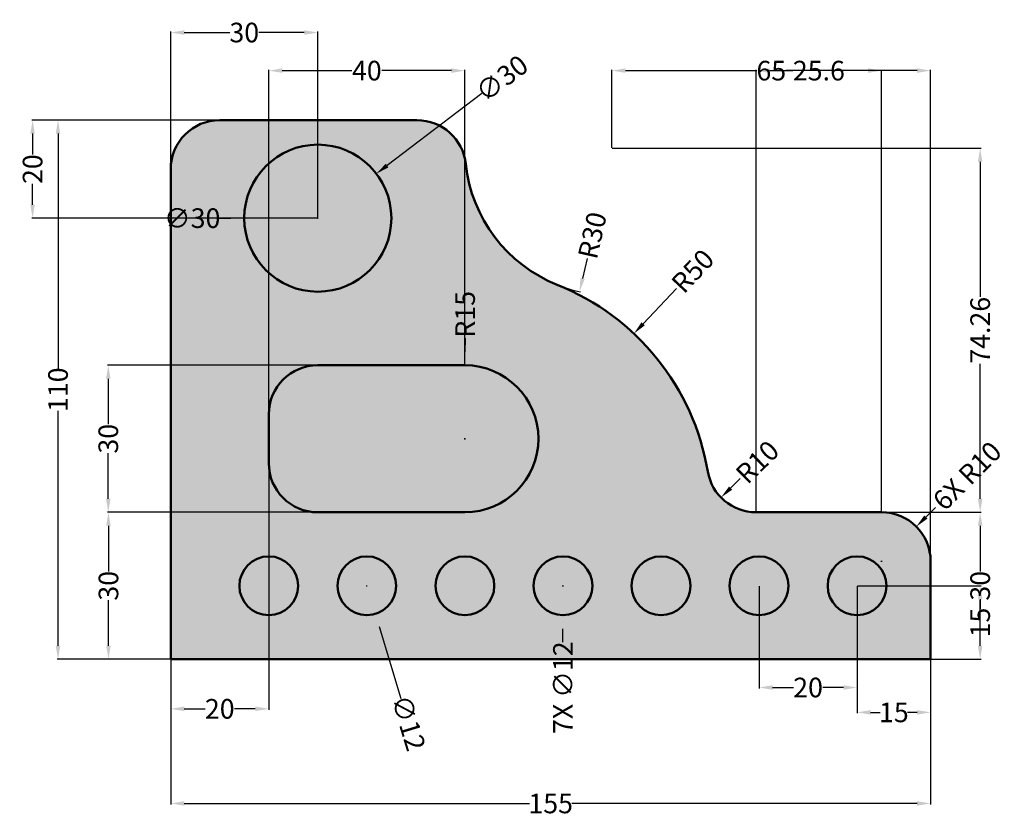
# Model space of a CAD drawing. Units: millimetres. Extents: x 347 to 548, y 156 to 318.
import ezdxf

# ---------------------------------------------------------------- set-up
doc = ezdxf.new("R2010")
doc.units = ezdxf.units.MM
doc.header["$MEASUREMENT"] = 0
doc.layers.add('M-DIMS', color=6, linetype='Continuous', lineweight=25)
doc.layers.add('M-OUTL', color=250, linetype='Continuous', lineweight=50)
doc.layers.add('M-HATC', color=252, linetype='Continuous', lineweight=18, true_color=0x939598)
doc.layers.add('M-HATC-OPENINGS', color=41, linetype='Continuous', lineweight=18, true_color=0xf4ee51)
doc.styles.get("Standard").update_dxf_attribs({"font": 'arial.ttf'})
doc.dimstyles.get("Standard").update_dxf_attribs({"dimtxt": 4, "dimasz": 2.75, "dimexe": 0.18, "dimexo": 0.0625, "dimgap": 0.09, "dimtad": 0, "dimdec": 0, "dimzin": 0, "dimdsep": 46, "dimtxsty": 'Standard', "dimcen": 0.09, "dimadec": 0, "dimazin": 0, "dimtfac": 1, "dimtdec": 0, "dimtofl": 0, "dimtmove": 0, "dimatfit": 3, "dimfxl": 1, "dimtolj": 1, "dimtzin": 0, "dimarcsym": 0})

# ---------------------------------------------------------------- blocks, each defined once
blk = doc.blocks.new('*D1')
at = {"layer": 'Defpoints', "color": 0, "transparency": 16777216}
for p in [(422.92, 217.89), (365.22, 187.89), (422.92, 187.89)]:
    blk.add_point(p, dxfattribs=at)
at = {"layer": 'M-DIMS', "color": 0, "lineweight": -2, "transparency": 16777216}
for p, q in [((422.85, 217.89), (365.04, 217.89)), ((365.22, 215.14), (365.22, 205.83)), ((365.22, 190.64), (365.22, 199.94)), ((422.85, 187.89), (365.04, 187.89))]:
    blk.add_line(p, q, dxfattribs=at)
at = {"layer": 'M-DIMS', "color": 0, "transparency": 16777216}
for points in [[(364.76, 215.14), (365.67, 215.14), (365.22, 217.89)], [(364.76, 190.64), (365.67, 190.64), (365.22, 187.89)]]:
    blk.add_solid(points, dxfattribs=at)
at = {"layer": 'M-DIMS', "color": 0, "transparency": 16777216, "insert": (365.22, 202.89), "char_height": 4, "attachment_point": 5, "rotation": 90}
blk.add_mtext('\\A1;30', dxfattribs=at)
blk = doc.blocks.new('*D2')
at = {"layer": 'Defpoints', "color": 0, "transparency": 16777216}
for p in [(365.18, 247.89), (422.92, 247.89), (422.92, 217.89)]:
    blk.add_point(p, dxfattribs=at)
at = {"layer": 'M-DIMS', "color": 0, "lineweight": -2, "transparency": 16777216}
for p, q in [((422.85, 247.89), (365, 247.89)), ((365.18, 245.14), (365.18, 235.83)), ((365.18, 220.64), (365.18, 229.94)), ((422.85, 217.89), (365, 217.89))]:
    blk.add_line(p, q, dxfattribs=at)
at = {"layer": 'M-DIMS', "color": 0, "transparency": 16777216}
for points in [[(364.72, 245.14), (365.64, 245.14), (365.18, 247.89)], [(364.72, 220.64), (365.64, 220.64), (365.18, 217.89)]]:
    blk.add_solid(points, dxfattribs=at)
at = {"layer": 'M-DIMS', "color": 0, "transparency": 16777216, "insert": (365.18, 232.89), "char_height": 4, "attachment_point": 5, "rotation": 90}
blk.add_mtext('\\A1;30', dxfattribs=at)
blk = doc.blocks.new('*D3')
at = {"layer": 'Defpoints', "color": 0, "transparency": 16777216}
for p in [(349.74, 297.89), (408.03, 297.89), (407.92, 277.89)]:
    blk.add_point(p, dxfattribs=at)
at = {"layer": 'M-DIMS', "color": 0, "lineweight": -2, "transparency": 16777216}
for p, q in [((407.97, 297.89), (349.56, 297.89)), ((349.74, 295.14), (349.74, 290.87)), ((349.74, 280.64), (349.74, 284.9)), ((407.85, 277.89), (349.56, 277.89))]:
    blk.add_line(p, q, dxfattribs=at)
at = {"layer": 'M-DIMS', "color": 0, "transparency": 16777216}
for points in [[(349.28, 295.14), (350.19, 295.14), (349.74, 297.89)], [(349.28, 280.64), (350.19, 280.64), (349.74, 277.89)]]:
    blk.add_solid(points, dxfattribs=at)
at = {"layer": 'M-DIMS', "color": 0, "transparency": 16777216, "insert": (349.74, 287.89), "char_height": 4, "attachment_point": 5, "rotation": 90}
blk.add_mtext('\\A1;20', dxfattribs=at)
blk = doc.blocks.new('*D4')
at = {"layer": 'Defpoints', "color": 0, "transparency": 16777216}
for p in [(407.92, 315.76), (377.92, 277.89), (407.92, 277.89)]:
    blk.add_point(p, dxfattribs=at)
at = {"layer": 'M-DIMS', "color": 0, "lineweight": -2, "transparency": 16777216}
for p, q in [((377.92, 277.95), (377.92, 315.94)), ((380.67, 315.76), (389.97, 315.76)), ((405.17, 315.76), (395.86, 315.76)), ((407.92, 277.95), (407.92, 315.94))]:
    blk.add_line(p, q, dxfattribs=at)
at = {"layer": 'M-DIMS', "color": 0, "transparency": 16777216}
for points in [[(380.67, 316.22), (380.67, 315.3), (377.92, 315.76)], [(405.17, 316.22), (405.17, 315.3), (407.92, 315.76)]]:
    blk.add_solid(points, dxfattribs=at)
at = {"layer": 'M-DIMS', "color": 0, "transparency": 16777216, "insert": (392.92, 315.76), "char_height": 4, "attachment_point": 5}
blk.add_mtext('\\A1;30', dxfattribs=at)
blk = doc.blocks.new('*D5')
at = {"layer": 'Defpoints', "color": 0, "transparency": 16777216}
for p in [(387.92, 297.89), (354.93, 187.89), (387.92, 187.89)]:
    blk.add_point(p, dxfattribs=at)
at = {"layer": 'M-DIMS', "color": 0, "lineweight": -2, "transparency": 16777216}
for p, q in [((387.85, 297.89), (354.75, 297.89)), ((354.93, 295.14), (354.93, 247.2)), ((354.93, 190.64), (354.93, 238.57)), ((387.85, 187.89), (354.75, 187.89))]:
    blk.add_line(p, q, dxfattribs=at)
at = {"layer": 'M-DIMS', "color": 0, "transparency": 16777216}
for points in [[(354.47, 295.14), (355.39, 295.14), (354.93, 297.89)], [(354.47, 190.64), (355.39, 190.64), (354.93, 187.89)]]:
    blk.add_solid(points, dxfattribs=at)
at = {"layer": 'M-DIMS', "color": 0, "transparency": 16777216, "insert": (354.93, 242.89), "char_height": 4, "attachment_point": 5, "rotation": 90}
blk.add_mtext('\\A1;110', dxfattribs=at)
blk = doc.blocks.new('*D6')
at = {"layer": 'Defpoints', "color": 0, "transparency": 16777216}
for p in [(419.86, 286.96), (395.97, 268.81)]:
    blk.add_point(p, dxfattribs=at)
at = {"layer": 'M-DIMS', "color": 0, "lineweight": -2, "transparency": 16777216}
for p, q in [((441.38, 303.31), (422.05, 288.63)), ((407.83, 277.89), (408.01, 277.89)), ((407.92, 277.8), (407.92, 277.98))]:
    blk.add_line(p, q, dxfattribs=at)
at = {"layer": 'M-DIMS', "color": 0, "transparency": 16777216}
blk.add_solid([(421.77, 288.99), (422.33, 288.26), (419.86, 286.96)], dxfattribs=at)
at = {"layer": 'M-DIMS', "color": 0, "transparency": 16777216, "insert": (445.46, 306.41), "char_height": 4, "attachment_point": 5, "rotation": 37.2288}
blk.add_mtext('\\A1;∅30', dxfattribs=at)
blk = doc.blocks.new('*D7')
at = {"layer": 'Defpoints', "color": 0, "transparency": 16777216}
for p in [(467.92, 292.15), (461.31, 262.88)]:
    blk.add_point(p, dxfattribs=at)
at = {"layer": 'M-DIMS', "color": 0, "lineweight": -2, "transparency": 16777216}
blk.add_line((462.84, 269.63), (461.92, 265.56), dxfattribs=at)
blk.add_arc((467.92, 292.15), 30, 248.2811, 257.6241, dxfattribs=at)
at = {"layer": 'M-DIMS', "color": 0, "transparency": 16777216}
blk.add_solid([(461.47, 265.67), (462.36, 265.46), (461.31, 262.88)], dxfattribs=at)
at = {"layer": 'M-DIMS', "color": 0, "transparency": 16777216, "insert": (463.91, 274.38), "char_height": 4, "attachment_point": 5, "rotation": 77.2804}
blk.add_mtext('\\A1;R30', dxfattribs=at)
blk = doc.blocks.new('*D8')
at = {"layer": 'Defpoints', "color": 0, "transparency": 16777216}
for p in [(472.39, 254.33), (438.16, 217.89)]:
    blk.add_point(p, dxfattribs=at)
at = {"layer": 'M-DIMS', "color": 0, "lineweight": -2, "transparency": 16777216}
for p, q in [((481.06, 263.56), (474.27, 256.33)), ((438.07, 217.89), (438.25, 217.89)), ((438.16, 217.8), (438.16, 217.98))]:
    blk.add_line(p, q, dxfattribs=at)
at = {"layer": 'M-DIMS', "color": 0, "transparency": 16777216}
blk.add_solid([(473.94, 256.65), (474.61, 256.02), (472.39, 254.33)], dxfattribs=at)
at = {"layer": 'M-DIMS', "color": 0, "transparency": 16777216, "insert": (484.39, 267.11), "char_height": 4, "attachment_point": 5, "rotation": 46.7913}
blk.add_mtext('\\A1;R50', dxfattribs=at)
blk = doc.blocks.new('*D9')
at = {"layer": 'Defpoints', "color": 0, "transparency": 16777216}
for p in [(497.32, 227.89), (490.16, 220.91)]:
    blk.add_point(p, dxfattribs=at)
at = {"layer": 'M-DIMS', "color": 0, "lineweight": -2, "transparency": 16777216}
blk.add_line((494.1, 224.75), (492.13, 222.83), dxfattribs=at)
at = {"layer": 'M-DIMS', "color": 0, "transparency": 16777216}
blk.add_solid([(491.81, 223.15), (492.45, 222.5), (490.16, 220.91)], dxfattribs=at)
at = {"layer": 'M-DIMS', "color": 0, "transparency": 16777216, "insert": (497.58, 228.14), "char_height": 4, "attachment_point": 5, "rotation": 44.268}
blk.add_mtext('\\A1;R10', dxfattribs=at)
blk = doc.blocks.new('*D10')
at = {"layer": 'Defpoints', "color": 0, "transparency": 16777216}
for p in [(497.92, 202.89), (517.92, 202.89), (517.92, 182.14)]:
    blk.add_point(p, dxfattribs=at)
at = {"layer": 'M-DIMS', "color": 0, "lineweight": -2, "transparency": 16777216}
for p, q in [((497.92, 202.82), (497.92, 181.96)), ((517.92, 202.82), (517.92, 181.96)), ((500.67, 182.14), (504.94, 182.14)), ((515.17, 182.14), (510.9, 182.14))]:
    blk.add_line(p, q, dxfattribs=at)
at = {"layer": 'M-DIMS', "color": 0, "transparency": 16777216}
for points in [[(500.67, 182.59), (500.67, 181.68), (497.92, 182.14)], [(515.17, 182.59), (515.17, 181.68), (517.92, 182.14)]]:
    blk.add_solid(points, dxfattribs=at)
at = {"layer": 'M-DIMS', "color": 0, "transparency": 16777216, "insert": (507.92, 182.14), "char_height": 4, "attachment_point": 5}
blk.add_mtext('\\A1;20', dxfattribs=at)
blk = doc.blocks.new('*D11')
at = {"layer": 'Defpoints', "color": 0, "transparency": 16777216}
for p in [(517.92, 202.89), (532.92, 202.89), (532.92, 177.06)]:
    blk.add_point(p, dxfattribs=at)
at = {"layer": 'M-DIMS', "color": 0, "lineweight": -2, "transparency": 16777216}
for p, q in [((517.92, 202.82), (517.92, 176.88)), ((532.92, 202.82), (532.92, 176.88)), ((520.67, 177.06), (522.64, 177.06)), ((530.17, 177.06), (528.2, 177.06))]:
    blk.add_line(p, q, dxfattribs=at)
at = {"layer": 'M-DIMS', "color": 0, "transparency": 16777216}
for points in [[(520.67, 177.52), (520.67, 176.6), (517.92, 177.06)], [(530.17, 177.52), (530.17, 176.6), (532.92, 177.06)]]:
    blk.add_solid(points, dxfattribs=at)
at = {"layer": 'M-DIMS', "color": 0, "transparency": 16777216, "insert": (525.42, 177.06), "char_height": 4, "attachment_point": 5}
blk.add_mtext('\\A1;15', dxfattribs=at)
blk = doc.blocks.new('*D12')
at = {"layer": 'Defpoints', "color": 0, "transparency": 16777216}
for p in [(377.92, 187.89), (532.92, 187.89), (532.92, 158.48)]:
    blk.add_point(p, dxfattribs=at)
at = {"layer": 'M-DIMS', "color": 0, "lineweight": -2, "transparency": 16777216}
for p, q in [((377.92, 187.82), (377.92, 158.3)), ((532.92, 187.82), (532.92, 158.3)), ((380.67, 158.48), (451.08, 158.48)), ((530.17, 158.48), (459.75, 158.48))]:
    blk.add_line(p, q, dxfattribs=at)
at = {"layer": 'M-DIMS', "color": 0, "transparency": 16777216}
for points in [[(380.67, 158.94), (380.67, 158.03), (377.92, 158.48)], [(530.17, 158.94), (530.17, 158.03), (532.92, 158.48)]]:
    blk.add_solid(points, dxfattribs=at)
at = {"layer": 'M-DIMS', "color": 0, "transparency": 16777216, "insert": (455.42, 158.48), "char_height": 4, "attachment_point": 5}
blk.add_mtext('\\A1;155', dxfattribs=at)
blk = doc.blocks.new('*D13')
at = {"layer": 'Defpoints', "color": 0, "transparency": 16777216}
for p in [(416.17, 208.63), (419.67, 197.15)]:
    blk.add_point(p, dxfattribs=at)
at = {"layer": 'M-DIMS', "color": 0, "lineweight": -2, "transparency": 16777216}
for p, q in [((417.83, 202.89), (418.01, 202.89)), ((417.92, 202.8), (417.92, 202.98)), ((424.95, 179.8), (420.47, 194.52))]:
    blk.add_line(p, q, dxfattribs=at)
at = {"layer": 'M-DIMS', "color": 0, "transparency": 16777216}
blk.add_solid([(420.91, 194.65), (420.03, 194.38), (419.67, 197.15)], dxfattribs=at)
at = {"layer": 'M-DIMS', "color": 0, "transparency": 16777216, "insert": (426.44, 174.91), "char_height": 4, "attachment_point": 5, "rotation": 286.9446}
blk.add_mtext('\\A1;∅12', dxfattribs=at)
blk = doc.blocks.new('FLANGE-HOLE-D12')
blk.add_circle((6, 6), 6)
blk = doc.blocks.new('*D15')
at = {"layer": 'Defpoints', "color": 0, "transparency": 16777216}
for p in [(517.92, 202.89), (532.92, 187.89), (543.02, 187.89)]:
    blk.add_point(p, dxfattribs=at)
at = {"layer": 'M-DIMS', "color": 0, "lineweight": -2, "transparency": 16777216}
for p, q in [((517.98, 202.89), (543.2, 202.89)), ((543.02, 200.14), (543.02, 198.17)), ((543.02, 190.64), (543.02, 192.61)), ((532.98, 187.89), (543.2, 187.89))]:
    blk.add_line(p, q, dxfattribs=at)
at = {"layer": 'M-DIMS', "color": 0, "transparency": 16777216}
for points in [[(542.56, 200.14), (543.48, 200.14), (543.02, 202.89)], [(542.56, 190.64), (543.48, 190.64), (543.02, 187.89)]]:
    blk.add_solid(points, dxfattribs=at)
at = {"layer": 'M-DIMS', "color": 0, "transparency": 16777216, "insert": (543.02, 195.39), "char_height": 4, "attachment_point": 5, "rotation": 90}
blk.add_mtext('\\A1;15', dxfattribs=at)
blk = doc.blocks.new('*D16')
at = {"layer": 'Defpoints', "color": 0, "transparency": 16777216}
for p in [(397.92, 227.89), (377.92, 187.89), (397.92, 177.79)]:
    blk.add_point(p, dxfattribs=at)
at = {"layer": 'M-DIMS', "color": 0, "lineweight": -2, "transparency": 16777216}
for p, q in [((397.92, 227.82), (397.92, 177.61)), ((377.92, 187.82), (377.92, 177.61)), ((380.67, 177.79), (384.94, 177.79)), ((395.17, 177.79), (390.9, 177.79))]:
    blk.add_line(p, q, dxfattribs=at)
at = {"layer": 'M-DIMS', "color": 0, "transparency": 16777216}
for points in [[(380.67, 178.25), (380.67, 177.33), (377.92, 177.79)], [(395.17, 178.25), (395.17, 177.33), (397.92, 177.79)]]:
    blk.add_solid(points, dxfattribs=at)
at = {"layer": 'M-DIMS', "color": 0, "transparency": 16777216, "insert": (387.92, 177.79), "char_height": 4, "attachment_point": 5}
blk.add_mtext('\\A1;20', dxfattribs=at)
blk = doc.blocks.new('*D17')
at = {"layer": 'Defpoints', "color": 0, "transparency": 16777216}
for p in [(437.92, 307.99), (437.92, 247.89), (397.92, 237.89)]:
    blk.add_point(p, dxfattribs=at)
at = {"layer": 'M-DIMS', "color": 0, "lineweight": -2, "transparency": 16777216}
for p, q in [((397.92, 237.95), (397.92, 308.17)), ((400.67, 307.99), (414.89, 307.99)), ((435.17, 307.99), (420.95, 307.99)), ((437.92, 247.95), (437.92, 308.17))]:
    blk.add_line(p, q, dxfattribs=at)
at = {"layer": 'M-DIMS', "color": 0, "transparency": 16777216}
for points in [[(400.67, 308.45), (400.67, 307.53), (397.92, 307.99)], [(435.17, 308.45), (435.17, 307.53), (437.92, 307.99)]]:
    blk.add_solid(points, dxfattribs=at)
at = {"layer": 'M-DIMS', "color": 0, "transparency": 16777216, "insert": (417.92, 307.99), "char_height": 4, "attachment_point": 5}
blk.add_mtext('\\A1;40', dxfattribs=at)
blk = doc.blocks.new('*D18')
at = {"layer": 'Defpoints', "color": 0, "transparency": 16777216}
for p in [(522.92, 217.89), (532.92, 187.89), (543.02, 187.89)]:
    blk.add_point(p, dxfattribs=at)
at = {"layer": 'M-DIMS', "color": 0, "lineweight": -2, "transparency": 16777216}
for p, q in [((522.98, 217.89), (543.2, 217.89)), ((543.02, 215.14), (543.02, 205.83)), ((543.02, 190.64), (543.02, 199.94)), ((532.98, 187.89), (543.2, 187.89))]:
    blk.add_line(p, q, dxfattribs=at)
at = {"layer": 'M-DIMS', "color": 0, "transparency": 16777216}
for points in [[(542.56, 215.14), (543.48, 215.14), (543.02, 217.89)], [(542.56, 190.64), (543.48, 190.64), (543.02, 187.89)]]:
    blk.add_solid(points, dxfattribs=at)
at = {"layer": 'M-DIMS', "color": 0, "transparency": 16777216, "insert": (543.02, 202.89), "char_height": 4, "attachment_point": 5, "rotation": 90}
blk.add_mtext('\\A1;30', dxfattribs=at)
blk = doc.blocks.new('*D19')
at = {"layer": 'Defpoints', "color": 0, "transparency": 16777216}
for p in [(522.92, 307.99), (497.32, 217.89), (522.92, 217.89)]:
    blk.add_point(p, dxfattribs=at)
at = {"layer": 'M-DIMS', "color": 0, "lineweight": -2, "transparency": 16777216}
for p, q in [((497.32, 217.95), (497.32, 308.17)), ((500.07, 307.99), (504.8, 307.99)), ((520.17, 307.99), (515.44, 307.99)), ((522.92, 217.95), (522.92, 308.17))]:
    blk.add_line(p, q, dxfattribs=at)
at = {"layer": 'M-DIMS', "color": 0, "transparency": 16777216}
for points in [[(500.07, 308.45), (500.07, 307.53), (497.32, 307.99)], [(520.17, 308.45), (520.17, 307.53), (522.92, 307.99)]]:
    blk.add_solid(points, dxfattribs=at)
at = {"layer": 'M-DIMS', "color": 0, "transparency": 16777216, "insert": (510.12, 307.99), "char_height": 4, "attachment_point": 5}
blk.add_mtext('\\A1;25.6', dxfattribs=at)
blk = doc.blocks.new('*D20')
at = {"layer": 'Defpoints', "color": 0, "transparency": 16777216}
for p in [(532.92, 307.99), (467.92, 292.15), (532.92, 207.89)]:
    blk.add_point(p, dxfattribs=at)
at = {"layer": 'M-DIMS', "color": 0, "lineweight": -2, "transparency": 16777216}
for p, q in [((467.92, 292.21), (467.92, 308.17)), ((470.67, 307.99), (497.44, 307.99)), ((530.17, 307.99), (503.4, 307.99)), ((532.92, 207.95), (532.92, 308.17))]:
    blk.add_line(p, q, dxfattribs=at)
at = {"layer": 'M-DIMS', "color": 0, "transparency": 16777216}
for points in [[(470.67, 308.45), (470.67, 307.53), (467.92, 307.99)], [(530.17, 308.45), (530.17, 307.53), (532.92, 307.99)]]:
    blk.add_solid(points, dxfattribs=at)
at = {"layer": 'M-DIMS', "color": 0, "transparency": 16777216, "insert": (500.42, 307.99), "char_height": 4, "attachment_point": 5}
blk.add_mtext('\\A1;65', dxfattribs=at)
blk = doc.blocks.new('*D21')
at = {"layer": 'Defpoints', "color": 0, "transparency": 16777216}
for p in [(467.92, 292.15), (522.92, 217.89), (543.02, 217.89)]:
    blk.add_point(p, dxfattribs=at)
at = {"layer": 'M-DIMS', "color": 0, "lineweight": -2, "transparency": 16777216}
for p, q in [((467.98, 292.15), (543.2, 292.15)), ((543.02, 289.4), (543.02, 261.84)), ((543.02, 220.64), (543.02, 248.2)), ((522.98, 217.89), (543.2, 217.89))]:
    blk.add_line(p, q, dxfattribs=at)
at = {"layer": 'M-DIMS', "color": 0, "transparency": 16777216}
for points in [[(542.56, 289.4), (543.48, 289.4), (543.02, 292.15)], [(542.56, 220.64), (543.48, 220.64), (543.02, 217.89)]]:
    blk.add_solid(points, dxfattribs=at)
at = {"layer": 'M-DIMS', "color": 0, "transparency": 16777216, "insert": (543.02, 255.02), "char_height": 4, "attachment_point": 5, "rotation": 90}
blk.add_mtext('\\A1;74.26', dxfattribs=at)
blk = doc.blocks.new('*D22')
at = {"layer": 'Defpoints', "color": 0, "transparency": 16777216}
for p in [(392.92, 277.89), (422.92, 277.89)]:
    blk.add_point(p, dxfattribs=at)
at = {"layer": 'M-DIMS', "color": 0, "lineweight": -2, "transparency": 16777216}
for p, q in [((387.42, 277.89), (390.17, 277.89)), ((407.83, 277.89), (408.01, 277.89)), ((407.92, 277.8), (407.92, 277.98))]:
    blk.add_line(p, q, dxfattribs=at)
at = {"layer": 'M-DIMS', "color": 0, "transparency": 16777216}
blk.add_solid([(390.17, 278.35), (390.17, 277.43), (392.92, 277.89)], dxfattribs=at)
at = {"layer": 'M-DIMS', "color": 0, "transparency": 16777216, "insert": (382.29, 277.89), "char_height": 4, "attachment_point": 5, "rotation": 0.0002}
blk.add_mtext('\\A1;∅30', dxfattribs=at)
blk = doc.blocks.new('*D23')
at = {"layer": 'Defpoints', "color": 0, "transparency": 16777216}
for p in [(437.94, 247.89), (437.92, 232.89)]:
    blk.add_point(p, dxfattribs=at)
at = {"layer": 'M-DIMS', "color": 0, "lineweight": -2, "transparency": 16777216}
for p, q in [((437.95, 253.39), (437.94, 250.64)), ((437.92, 232.8), (437.92, 232.98)), ((437.83, 232.89), (438.01, 232.89))]:
    blk.add_line(p, q, dxfattribs=at)
at = {"layer": 'M-DIMS', "color": 0, "transparency": 16777216}
blk.add_solid([(437.49, 250.64), (438.4, 250.64), (437.94, 247.89)], dxfattribs=at)
at = {"layer": 'M-DIMS', "color": 0, "transparency": 16777216, "insert": (437.96, 258.27), "char_height": 4, "attachment_point": 5, "rotation": 89.9138}
blk.add_mtext('\\A1;R15', dxfattribs=at)
blk = doc.blocks.new('*D24')
at = {"layer": 'Defpoints', "color": 0, "transparency": 16777216}
for p in [(529.99, 214.96), (522.92, 207.89)]:
    blk.add_point(p, dxfattribs=at)
at = {"layer": 'M-DIMS', "color": 0, "lineweight": -2, "transparency": 16777216}
for p, q in [((533.88, 218.85), (531.93, 216.9)), ((522.83, 207.89), (523.01, 207.89)), ((522.92, 207.8), (522.92, 207.98))]:
    blk.add_line(p, q, dxfattribs=at)
at = {"layer": 'M-DIMS', "color": 0, "transparency": 16777216}
blk.add_solid([(531.61, 217.23), (532.26, 216.58), (529.99, 214.96)], dxfattribs=at)
at = {"layer": 'M-DIMS', "color": 0, "transparency": 16777216, "insert": (540.36, 225.33), "char_height": 4, "attachment_point": 5, "rotation": 45.0015}
blk.add_mtext('\\A1;6X R10', dxfattribs=at)
blk = doc.blocks.new('*D25')
at = {"layer": 'Defpoints', "color": 0, "transparency": 16777216}
for p in [(457.92, 208.89), (457.92, 196.89)]:
    blk.add_point(p, dxfattribs=at)
at = {"layer": 'M-DIMS', "color": 0, "lineweight": -2, "transparency": 16777216}
for p, q in [((457.83, 202.89), (458.01, 202.89)), ((457.92, 202.8), (457.92, 202.98)), ((457.92, 191.39), (457.92, 194.14))]:
    blk.add_line(p, q, dxfattribs=at)
at = {"layer": 'M-DIMS', "color": 0, "transparency": 16777216}
blk.add_solid([(457.46, 194.14), (458.38, 194.14), (457.92, 196.89)], dxfattribs=at)
at = {"layer": 'M-DIMS', "color": 0, "transparency": 16777216, "insert": (457.92, 182.1), "char_height": 4, "attachment_point": 5, "rotation": 89.996}
blk.add_mtext('\\A1;7X ∅12', dxfattribs=at)

msp = doc.modelspace()

# ---------------------------------------------------------------- hatches: boundary and pattern name
at = {"layer": 'M-HATC'}
h = msp.add_hatch(color=256, dxfattribs=at)
h.dxf.hatch_style = 1
h.paths.add_polyline_path([(456.758, 264.299, -0.2775575), (438.088, 288.952, 0.3833025), (428.145, 297.887), (387.917, 297.887, 0.4142136), (377.917, 287.887), (377.917, 187.887), (397.917, 187.887), (532.917, 187.887), (532.917, 207.887, 0.4142136), (522.917, 217.887), (497.319, 217.887, -0.3659774), (487.459, 226.22, 0.261262)])
h.paths.add_polyline_path([(407.917, 247.887), (437.917, 247.887, -1), (437.917, 217.887), (407.917, 217.887, -0.4142136), (397.917, 227.887), (397.917, 237.887, -0.4142136)], flags=16)
h.paths.add_polyline_path([(392.917, 277.887, -1), (422.917, 277.887, -1)], flags=16)
h.paths.add_polyline_path([(403.917, 202.887, -1), (391.917, 202.887, -1)], flags=16)
h.paths.add_polyline_path([(423.917, 202.887, -1), (411.917, 202.887, -1)], flags=16)
h.paths.add_polyline_path([(443.917, 202.887, -1), (431.917, 202.887, -1)], flags=16)
h.paths.add_polyline_path([(463.917, 202.887, -1), (451.917, 202.887, -1)], flags=16)
h.paths.add_polyline_path([(483.917, 202.887, -1), (471.917, 202.887, -1)], flags=16)
h.paths.add_polyline_path([(503.917, 202.887, -1), (491.917, 202.887, -1)], flags=16)
h.paths.add_polyline_path([(523.917, 202.887, -1), (511.917, 202.887, -1)], flags=16)
at = {"layer": 'M-HATC-OPENINGS'}
h = msp.add_hatch(color=256, dxfattribs=at)
h.dxf.hatch_style = 1
h.paths.add_polyline_path([(422.917, 277.887, 1), (392.917, 277.887, 1)])
h.paths.add_polyline_path([(437.917, 247.887), (407.917, 247.887, 0.4142136), (397.917, 237.887), (397.917, 232.887), (397.917, 227.887, 0.4142136), (407.917, 217.887), (437.917, 217.887, 1)])
h.paths.add_polyline_path([(391.917, 202.887, 1), (403.917, 202.887, 1)])
h.paths.add_polyline_path([(423.917, 202.887, 1), (411.917, 202.887, 1)])
h.paths.add_polyline_path([(443.917, 202.887, 1), (431.917, 202.887, 1)])
h.paths.add_polyline_path([(451.917, 202.887, 1), (463.917, 202.887, 1)])
h.paths.add_polyline_path([(483.917, 202.887, 1), (471.917, 202.887, 1)])
h.paths.add_polyline_path([(503.917, 202.887, 1), (491.917, 202.887, 1)])
h.paths.add_polyline_path([(523.917, 202.887, 1), (511.917, 202.887, 1)])

# ---------------------------------------------------------------- linework, layer by layer
at = {"layer": 'M-OUTL'}
for p, q in [((387.917, 297.887), (428.145, 297.887)), ((377.917, 187.887), (377.917, 287.887)), ((377.917, 287.887), (377.917, 187.887)), ((407.917, 247.887), (437.917, 247.887)), ((397.917, 232.887), (397.917, 237.887)), ((397.917, 227.887), (397.917, 237.887)), ((437.917, 217.887), (407.917, 217.887)), ((407.917, 217.887), (437.917, 217.887)), ((497.319, 217.887), (522.917, 217.887)), ((532.917, 187.887), (532.917, 207.887)), ((377.917, 187.887), (532.917, 187.887))]:
    msp.add_line(p, q, dxfattribs=at)
msp.add_circle((407.917, 277.887), 15, dxfattribs=at)
for centre, radius, start, end in [((387.917, 287.887), 10, 90, 180), ((428.145, 287.887), 10, 6.11219, 90), ((467.917, 292.146), 30, 186.11219, 248.16177), ((438.158, 217.887), 50, 9.59407, 68.16177), ((407.917, 237.887), 10, 90, 180), ((437.917, 232.887), 15, 270, 90), ((407.917, 227.887), 10, 180, 270), ((497.319, 227.887), 10, 189.59407, 270), ((522.917, 207.887), 10, 0, 90)]:
    msp.add_arc(centre, radius, start, end, dxfattribs=at)

# ---------------------------------------------------------------- block references
for p in [(391.917, 196.887), (411.917, 196.887), (431.917, 196.887), (451.917, 196.887), (471.917, 196.887), (491.917, 196.887), (511.917, 196.887)]:
    msp.add_blockref('FLANGE-HOLE-D12', p, dxfattribs=at)

# ---------------------------------------------------------------- dimensions: what is measured, and where the dimension line sits
at = {"layer": 'M-DIMS'}
for base, p1, p2, override, picture, middle in [((407.917, 315.757), (377.917, 277.887), (407.917, 277.887), {"dimclrd": 0, "dimclre": 0, "dimclrt": 0}, '*D4', (392.917, 315.757)), ((437.917, 307.987), (397.917, 237.887), (437.917, 247.887), {"dimdec": 0, "dimlfac": 1, "dimrnd": 0, "dimzin": 0, "dimdsep": 46, "dimlunit": 2}, '*D17', (417.917, 307.987)), ((532.917, 307.987), (467.917, 292.146), (532.917, 207.887), {"dimdec": 0, "dimlfac": 1, "dimrnd": 0, "dimzin": 0, "dimdsep": 46, "dimlunit": 2}, '*D20', (500.417, 307.987)), ((522.917, 307.987), (497.319, 217.887), (522.917, 217.887), {"dimdec": 1, "dimlfac": 1, "dimrnd": 0, "dimzin": 0, "dimdsep": 46, "dimlunit": 2}, '*D19', (510.118, 307.987)), ((397.917, 177.787), (377.917, 187.887), (397.917, 227.887), {"dimdec": 0, "dimlfac": 1, "dimrnd": 0, "dimzin": 0, "dimdsep": 46, "dimlunit": 2}, '*D16', (387.917, 177.787)), ((517.917, 182.136), (497.917, 202.887), (517.917, 202.887), {"dimclrd": 0, "dimclre": 0, "dimclrt": 0}, '*D10', (507.917, 182.136)), ((532.917, 177.061), (517.917, 202.887), (532.917, 202.887), {"dimclrd": 0, "dimclre": 0, "dimclrt": 0}, '*D11', (525.417, 177.061)), ((532.917, 158.484), (377.917, 187.887), (532.917, 187.887), {"dimclrd": 0, "dimclre": 0, "dimclrt": 0}, '*D12', (455.417, 158.484))]:
    dim = msp.add_linear_dim(base=base, p1=p1, p2=p2, dimstyle='Standard', override=override, dxfattribs=at)
    dim.commit()
    dim.dimension.update_dxf_attribs({"geometry": picture, "text_midpoint": middle})
for p1, p2, override, picture, middle in [((395.974, 268.812), (419.861, 286.962), {"dimclrd": 0, "dimclre": 0, "dimclrt": 0}, '*D6', (445.458, 306.412)), ((422.917, 277.887), (392.917, 277.887), {"dimdec": 0, "dimlfac": 1, "dimrnd": 0, "dimzin": 0, "dimdsep": 46, "dimlunit": 2}, '*D22', (382.293, 277.887)), ((416.169, 208.627), (419.666, 197.148), {"dimclrd": 0, "dimclre": 0, "dimclrt": 0}, '*D13', (426.441, 174.91))]:
    dim = msp.add_diameter_dim_2p(p1=p1, p2=p2, dimstyle='Standard', override=override, dxfattribs=at)
    dim.commit()
    dim.dimension.update_dxf_attribs({"geometry": picture, "text_midpoint": middle, "dimtype": 163})
for base, p1, p2, override, picture, middle in [((349.736, 297.887), (407.917, 277.887), (408.031, 297.887), {"dimclrd": 0, "dimclre": 0, "dimclrt": 0}, '*D3', (349.736, 287.887)), ((354.928, 187.887), (387.917, 297.887), (387.917, 187.887), {"dimclrd": 0, "dimclre": 0, "dimclrt": 0}, '*D5', (354.928, 242.887)), ((543.017, 217.887), (467.917, 292.146), (522.917, 217.887), {"dimdec": 2, "dimlfac": 1, "dimrnd": 0, "dimzin": 0, "dimdsep": 46, "dimlunit": 2}, '*D21', (543.017, 255.017)), ((365.179, 247.887), (422.917, 217.887), (422.917, 247.887), {"dimclrd": 0, "dimclre": 0, "dimclrt": 0}, '*D2', (365.179, 232.887)), ((365.215, 187.887), (422.917, 217.887), (422.917, 187.887), {"dimclrd": 0, "dimclre": 0, "dimclrt": 0}, '*D1', (365.215, 202.887)), ((543.017, 187.887), (522.917, 217.887), (532.917, 187.887), {"dimdec": 0, "dimlfac": 1, "dimrnd": 0, "dimzin": 0, "dimdsep": 46, "dimlunit": 2}, '*D18', (543.017, 202.887)), ((543.017, 187.887), (517.917, 202.887), (532.917, 187.887), {"dimdec": 0, "dimlfac": 1, "dimrnd": 0, "dimzin": 0, "dimdsep": 46, "dimlunit": 2}, '*D15', (543.017, 195.387))]:
    dim = msp.add_linear_dim(base=base, p1=p1, p2=p2, angle=90, dimstyle='Standard', override=override, dxfattribs=at)
    dim.commit()
    dim.dimension.update_dxf_attribs({"geometry": picture, "text_midpoint": middle})
for center, mpoint, picture, middle in [((467.917, 292.146), (461.312, 262.882), '*D7', (463.906, 274.375)), ((438.158, 217.887), (472.391, 254.33), '*D8', (484.392, 267.106)), ((497.319, 227.887), (490.158, 220.907), '*D9', (497.579, 228.14))]:
    dim = msp.add_radius_dim(center=center, mpoint=mpoint, dimstyle='Standard', override={"dimclrd": 0, "dimclre": 0, "dimclrt": 0}, dxfattribs=at)
    dim.commit()
    dim.dimension.update_dxf_attribs({"geometry": picture, "text_midpoint": middle, "dimtype": 164})
dim = msp.add_radius_dim(center=(437.917, 232.887), mpoint=(437.94, 247.887), dimstyle='Standard', override={"dimdec": 0, "dimlfac": 1, "dimrnd": 0, "dimzin": 0, "dimdsep": 46, "dimlunit": 2}, dxfattribs=at)
dim.commit()
dim.dimension.update_dxf_attribs({"geometry": '*D23', "text_midpoint": (437.956, 258.271)})
dim = msp.add_radius_dim(center=(522.917, 207.887), mpoint=(529.988, 214.958), text='6X <>', dimstyle='Standard', override={"dimdec": 0, "dimlfac": 1, "dimrnd": 0, "dimzin": 0, "dimdsep": 46, "dimlunit": 2}, dxfattribs=at)
dim.commit()
dim.dimension.update_dxf_attribs({"geometry": '*D24', "text_midpoint": (540.362, 225.332)})
dim = msp.add_diameter_dim_2p(p1=(457.918, 208.887), p2=(457.917, 196.887), text='7X <>', dimstyle='Standard', override={"dimdec": 0, "dimlfac": 1, "dimrnd": 0, "dimzin": 0, "dimdsep": 46, "dimlunit": 2}, dxfattribs=at)
dim.commit()
dim.dimension.update_dxf_attribs({"geometry": '*D25', "text_midpoint": (457.916, 182.102), "dimtype": 163})

doc.saveas('drawing.dxf')
